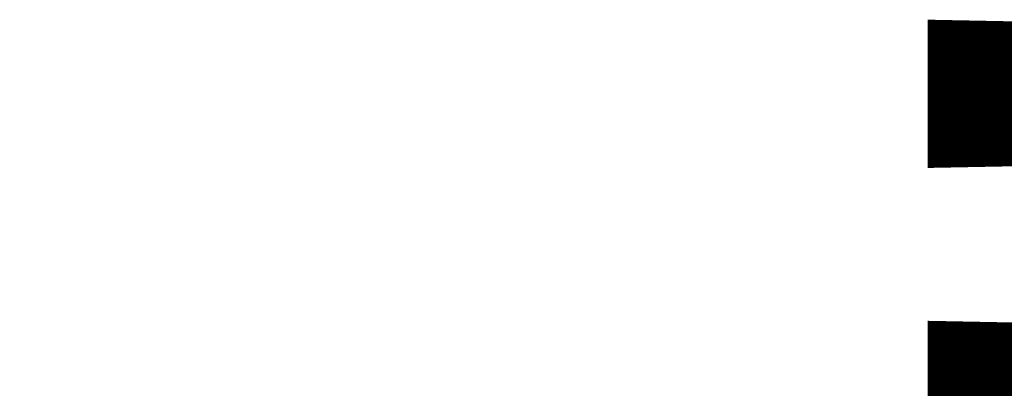
# Model space of a CAD drawing. Units: inches. Extents: x 597 to 1323, y 1833 to 2686.
# Tile 9 of 10: x 1100.86 to 1116.23, y 2509.42 to 2515.18. Entities that reach past the tile are written whole.
import ezdxf

# ---------------------------------------------------------------- set-up
doc = ezdxf.new("R2010")
doc.units = ezdxf.units.IN
doc.layers.add('A-ANNO-DIMS', color=2, linetype='Continuous', lineweight=18)
doc.styles.get("Standard").update_dxf_attribs({"font": 'arial.ttf'})
doc.dimstyles.new('ISO-25', dxfattribs={"dimtxt": 17.5, "dimasz": 2.5, "dimexe": 0, "dimexo": 0, "dimtad": 1, "dimdec": 1, "dimlunit": 3, "dimtxsty": 'Standard', "dimblk": 'OPEN90', "dimcen": 2.5, "dimadec": 0, "dimazin": 0, "dimtfac": 1, "dimtdec": 1, "dimtmove": 0, "dimatfit": 3, "dimfxl": 0, "dimfxlon": 1, "dimarcsym": 0})

# ---------------------------------------------------------------- blocks, each defined once
blk = doc.blocks.new('_Open90')
at = {"color": 0, "linetype": 'ByBlock', "lineweight": -2}
for p, q in [((-0.5, 0.5), (0, 0)), ((0, 0), (-1, 0)), ((0, 0), (-0.5, -0.5))]:
    blk.add_line(p, q, dxfattribs=at)
blk = doc.blocks.new('*D64')
at = {"layer": 'A-ANNO-DIMS', "color": 0, "lineweight": -2, "transparency": 16777216}
for p, q in [((1136.636, 2423.611), (1136.636, 2514.646)), ((1136.636, 2384.76), (1136.636, 2421.111))]:
    blk.add_line(p, q, dxfattribs=at)
at = {"layer": 'Defpoints', "color": 0, "transparency": 16777216}
for p in [(1107.886, 2423.611), (1136.636, 2423.611), (1107.886, 2382.26)]:
    blk.add_point(p, dxfattribs=at)
at = {"layer": 'A-ANNO-DIMS', "color": 0, "lineweight": -2, "transparency": 16777216, "xscale": 2.5, "yscale": 2.5, "zscale": 2.5}
for p, rotation in [((1136.636, 2423.611), 90), ((1136.636, 2382.26), 270)]:
    blk.add_blockref('_Open90', p, dxfattribs=dict(at, rotation=rotation))
at = {"layer": 'A-ANNO-DIMS', "color": 0, "transparency": 16777216, "insert": (1126.957, 2470.378), "char_height": 17.5, "attachment_point": 5, "rotation": 90}
blk.add_mtext('3\'-5 1/2"', dxfattribs=at)

msp = doc.modelspace()

# ---------------------------------------------------------------- dimensions: what is measured, and where the dimension line sits
at = {"layer": 'A-ANNO-DIMS'}
dim = msp.add_linear_dim(base=(1136.636, 2423.611), p1=(1107.886, 2382.26), p2=(1107.886, 2423.611), angle=90, dimstyle='ISO-25', override={"dimdec": 1, "dimlfac": 1, "dimrnd": 0, "dimzin": 1, "dimdsep": 46, "dimlunit": 4, "dimfrac": 2}, dxfattribs=at)
dim.commit()
dim.dimension.update_dxf_attribs({"geometry": '*D64', "text_midpoint": (1126.957, 2470.378)})

doc.saveas('drawing.dxf')
